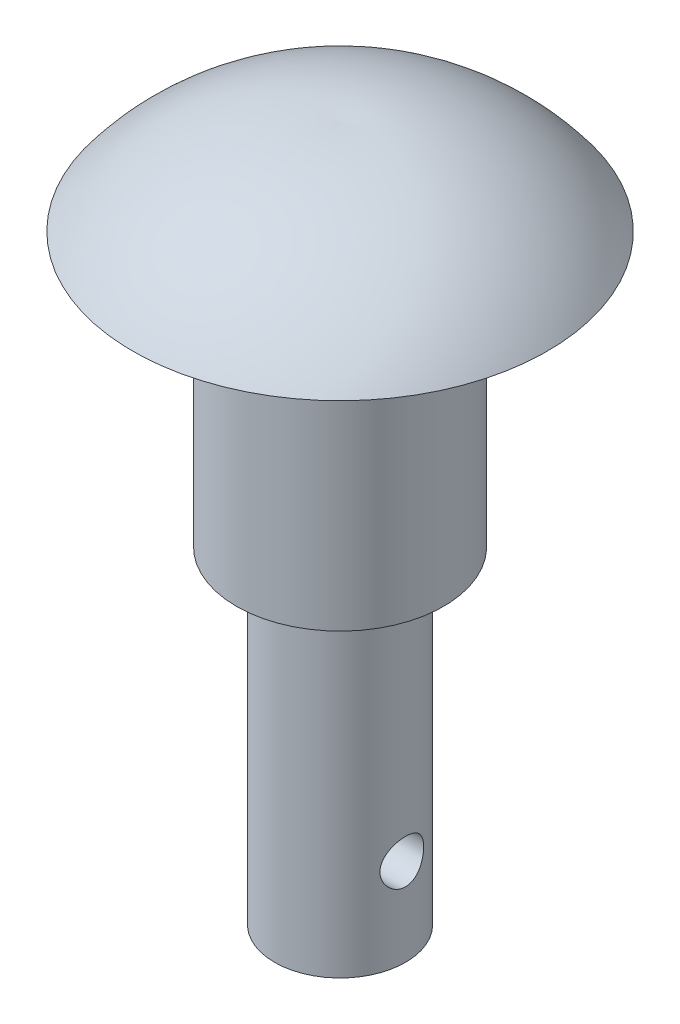
from build123d import *

# Parameters (mm, degrees)
SHAFT_PROFILE_12_R   = 6
SHAFT_12_DEPTH       = 30
COLLAR_PROFILE_19_R  = 9.5
COLLAR_19_DEPTH      = 25
CROSS_HOLE_PROFILE_R = 2
CROSS_HOLE_DEPTH     = 12.5


with BuildPart() as part:
    # Shaft Profile Ø12 → Shaft Ø12 (new body)
    with BuildSketch(Plane(origin=(0, 0, 0), x_dir=(1, 0, 0), z_dir=(0, 1, 0))):
        with Locations(Location((0, 0, 0), (0, 0, 270))):
            Circle(SHAFT_PROFILE_12_R)
    extrude(amount=SHAFT_12_DEPTH)

    # Collar Profile Ø19 → Collar Ø19 (add)
    with BuildSketch(Plane(origin=(0, 30, 0), x_dir=(1, 0, 0), z_dir=(0, 1, 0))):
        with Locations(Location((0, 0, 0), (0, 0, 270))):
            Circle(COLLAR_PROFILE_19_R)
    extrude(amount=COLLAR_19_DEPTH)

    # Dome Head Profile → Dome Head (revolve)
    with BuildSketch(Plane(origin=(0, 0, 0), x_dir=(0, 0, -1), z_dir=(1, 0, 0))):
        with BuildLine():
            Line((0, 55), (-19, 55))
            ThreePointArc((-19, 55), (-10.604187915, 61.769260733), (0, 63.734903146))
            Line((0, 63.734903146), (0, 55))
        make_face()
    revolve(axis=Axis((0, 55, 0), (0, 1, 0)))

    # Cross Hole Profile → Cross Hole (cut, symmetric)
    with BuildSketch(Plane(origin=(0, 0, 0), x_dir=(0, 0, -1), z_dir=(1, 0, 0))):
        with Locations((0, 8)):
            Circle(CROSS_HOLE_PROFILE_R)
    extrude(amount=CROSS_HOLE_DEPTH, both=True, mode=Mode.SUBTRACT)


solid = part.part
